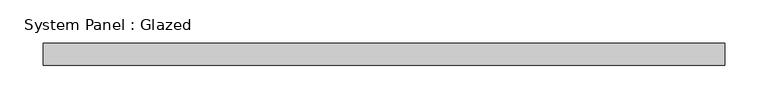
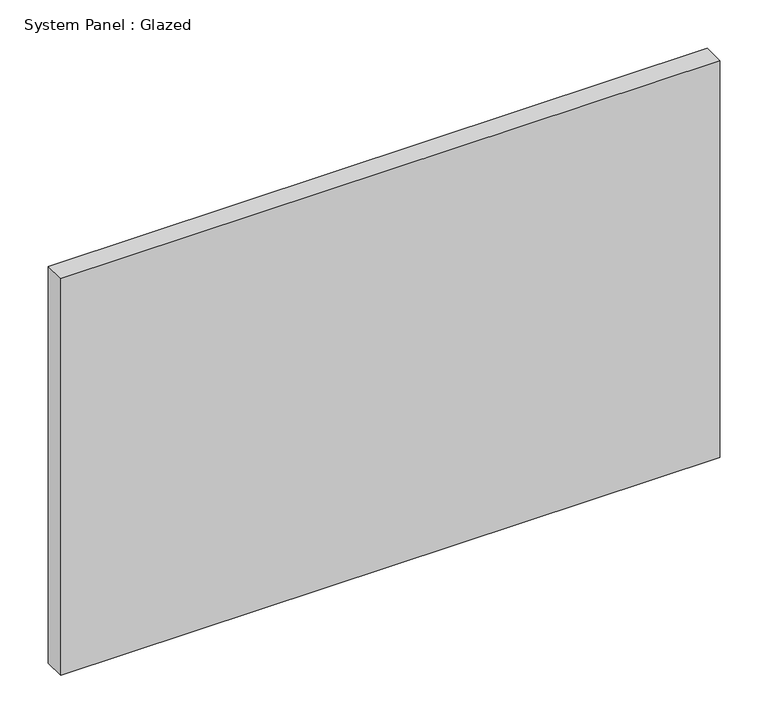
"""IFC4 building model written with IfcOpenShell, lengths in millimetres: plate geometry, System Panel : Glazed."""

from ifc_helpers import new_model, si_unit, origin, origin_with_axes, place, context, project, spatial, polyline, outline, extrude, source, transform, mapped, element, save


def system_panel_glazed_c2282f98(model_context):
    return source(origin(), model_context, "Body", "SweptSolid", [
        extrude(outline(polyline([(393.7, 19.05), (-393.7, 19.05), (-393.7, 44.45), (393.7, 44.45), (393.7, 19.05)])), origin_with_axes(), (0.0, 0.0, 1.0), 501.6559963),
    ])


if __name__ == "__main__":
    model = new_model("IFC4")
    model_context = context("Model", 3, world=origin())
    ifc_project = project(units=[si_unit("LENGTHUNIT", "METRE", prefix="MILLI")], contexts=[model_context])
    site = spatial("IfcSite", under=ifc_project)
    building = spatial("IfcBuilding", under=site)
    placement = place(None, origin())
    system_panel_glazed_shape = system_panel_glazed_c2282f98(model_context)
    element("IfcPlate", 1, ObjectType="System Panel : Glazed", at=placement, inside=building, context=model_context, shape_type="MappedRepresentation", body=[
        mapped(system_panel_glazed_shape, transform((0.0, 0.0, 0.0), x_axis=(1.0, 0.0, 0.0), y_axis=(0.0, 1.0, 0.0), z_axis=(0.0, 0.0, 1.0))),
    ])
    save(model, "model.ifc")

# Revit data of these elements
# Type "System Panel : Glazed"
#   Construction Type Id = "GSP4R"
#   Analytic Construction = "1/8 in Pilkington single glazing"
#   Visual Light Transmittance = 0.9
#   Solar Heat Gain Coefficient = 0.86
#   Heat Transfer Coefficient (U) = 1.18115 BTU/(h·ft²·°F)
#   Define Thermal Properties by = 1
# Element 1 (IfcPlate, "System Panel : Glazed")
#   Materials on its faces: "Glass"
# Materials
#   "Glass": class "Glass", colour RGB 0 128 192, transparency 0.75, Description = "Soda Lime Glass", Cost = 0
